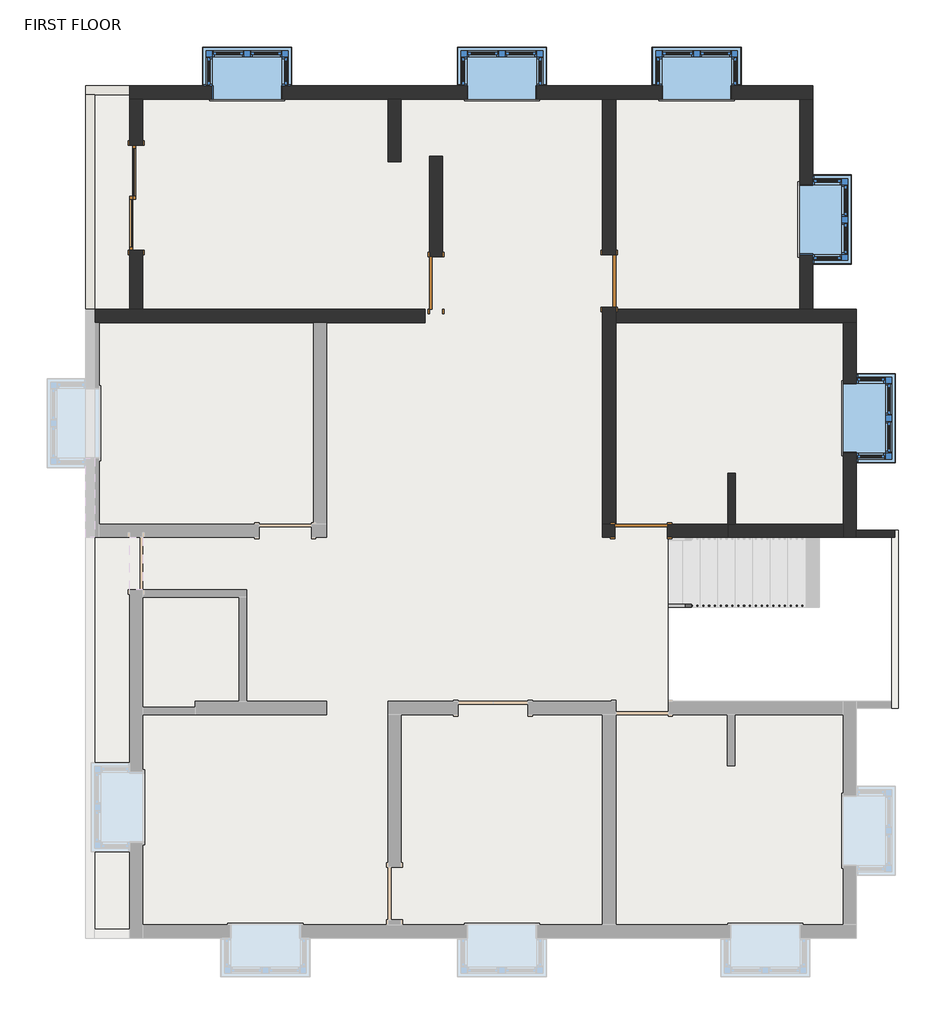
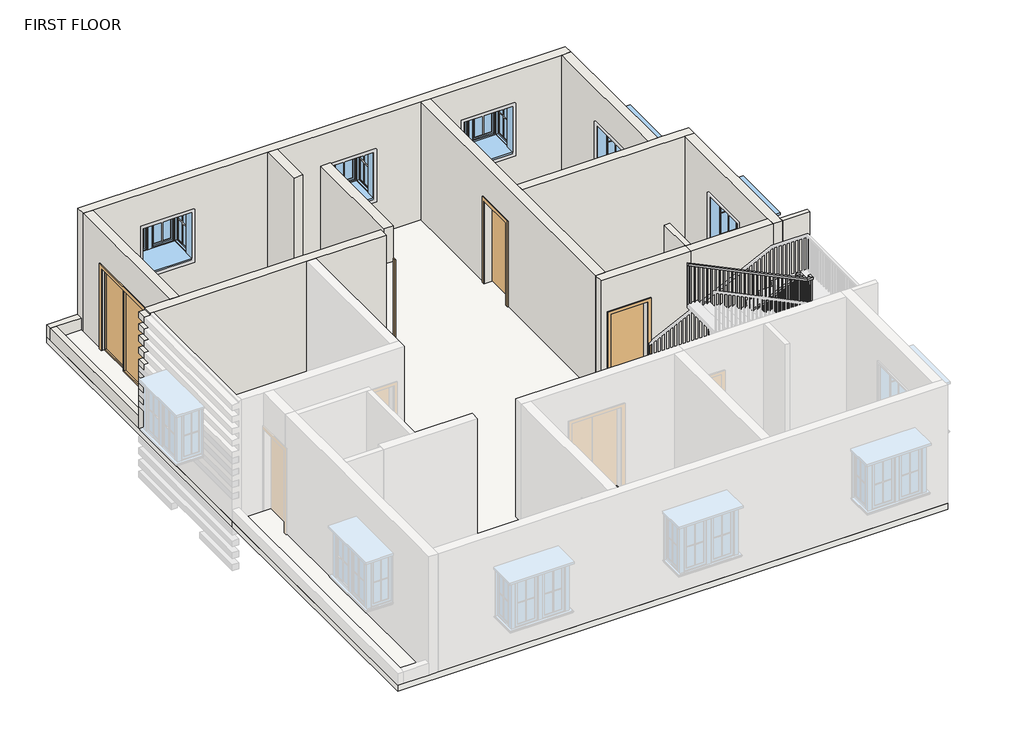
# One storey, part 2 of 6: 15 walls, 5 windows, 4 doors, 1 railing, 1 slab.
"""IFC4 building model written with IfcOpenShell, lengths in millimetres."""

from ifc_helpers import new_model, si_unit, frame, origin, place, context, project, spatial, polyline, outline, extrude, faceted_brep, transform, mapped, element, save
from components import door_d4d75d1e, door_a90ba1ad, door_0ca8825f, window_bay_casement_box_90_degree_angle_4_x4_x2_07b705a1

model = new_model("IFC4")

# Units and contexts
model_context = context("Model", 3, world=origin())
ifc_project = project(units=[si_unit("LENGTHUNIT", "METRE", prefix="MILLI")], contexts=[model_context])

# Site, building, storey
site = spatial("IfcSite", under=ifc_project)
building = spatial("IfcBuilding", under=site)
storey = spatial("IfcBuildingStorey", under=building, Name="FIRST FLOOR", Elevation=3200.4)

# Doors
placement = place(None, origin())
door_shape = door_d4d75d1e(model_context)
element("IfcDoor", 1, ObjectType="Door-Double-Sliding : 72\" x 84\"", at=placement, inside=storey, context=model_context, shape_type="MappedRepresentation", body=[
    mapped(door_shape, transform((-6005.0415084, 6126.233346, 3200.4), x_axis=(0.0, 1.0, 0.0), y_axis=(-1.0, 0.0, 0.0), z_axis=(0.0, 0.0, 1.0))),
])
door_2_shape = door_a90ba1ad(model_context)
element("IfcDoor", 2, ObjectType="Single-Flush : 36\" x 84\"", at=placement, inside=storey, context=model_context, shape_type="MappedRepresentation", body=[
    mapped(door_2_shape, transform((2656.3584916, 335.033346, 3200.4), x_axis=(-1.0, 0.0, 0.0), y_axis=(0.0, -1.0, 0.0), z_axis=(0.0, 0.0, 1.0))),
])
element("IfcDoor", 3, ObjectType="Single-Flush : 36\" x 84\"", at=placement, inside=storey, context=model_context, shape_type="MappedRepresentation", body=[
    mapped(door_2_shape, transform((-918.5024437, 4640.333346, 3200.4), x_axis=(0.0, -1.0, 0.0), y_axis=(1.0, 0.0, 0.0), z_axis=(0.0, 0.0, 1.0))),
])
door_3_shape = door_0ca8825f(model_context)
element("IfcDoor", 4, ObjectType="Single-Flush : 36\" x 84\"", at=placement, inside=storey, context=model_context, shape_type="MappedRepresentation", body=[
    mapped(door_3_shape, transform((2097.5584916, 4678.433346, 3200.4), x_axis=(0.0, -1.0, 0.0), y_axis=(1.0, 0.0, 0.0), z_axis=(0.0, 0.0, 1.0))),
])

# Railing
element("IfcRailing", 5, ObjectType="Handrail - Rectangular", at=placement, inside=storey, context=model_context, shape_type="SolidModel", body=[
    faceted_brep([(3126.2584916, -947.666654, 4260.2727273), (3126.2584916, -947.666654, 4203.7956113), (3126.2584916, -998.466654, 4203.7956113), (3126.2584916, -998.466654, 4260.2727273), (6044.5829507, -947.666654, 5677.9823634), (6095.3829507, -947.666654, 5646.1836718), (6095.3829507, -998.466654, 5646.1836718), (6044.5829507, -998.466654, 5677.9823634), (6044.5829507, -947.666654, 5715.0), (6095.3829507, -947.666654, 5664.2), (6095.3829507, -998.466654, 5664.2), (6044.5829507, -998.466654, 5715.0), (6171.5829507, -947.666654, 5715.0), (6171.5829507, -947.666654, 5664.2), (6120.7829507, -998.466654, 5664.2), (6120.7829507, -998.466654, 5715.0), (6171.5829507, -1074.666654, 5715.0), (6171.5829507, -1074.666654, 5664.2), (6120.7829507, -1074.666654, 5664.2), (6120.7829507, -1074.666654, 5715.0), (6171.5829507, -1341.366654, 5715.0), (6171.5829507, -1392.166654, 5664.2), (6120.7829507, -1392.166654, 5664.2), (6120.7829507, -1341.366654, 5715.0), (6171.5829507, -1341.366654, 5897.4903639), (6171.5829507, -1392.166654, 5846.6903639), (6120.7829507, -1392.166654, 5846.6903639), (6120.7829507, -1341.366654, 5897.4903639), (6171.5829507, -1468.366654, 5897.4903639), (6171.5829507, -1468.366654, 5846.6903639), (6120.7829507, -1417.566654, 5846.6903639), (6120.7829507, -1417.566654, 5897.4903639), (6044.5829507, -1468.366654, 5897.4903639), (6032.8967309, -1468.366654, 5846.6903639), (6032.8967309, -1417.566654, 5846.6903639), (6044.5829507, -1417.566654, 5897.4903639), (3126.2584916, -1468.366654, 7315.2), (3126.2584916, -1417.566654, 7315.2), (3126.2584916, -1417.566654, 7258.722884), (3126.2584916, -1468.366654, 7258.722884)], [[[0, 1, 2, 3]], [[1, 0, 4, 5]], [[2, 1, 5, 6]], [[3, 2, 6, 7]], [[0, 3, 7, 4]], [[5, 4, 8, 9]], [[6, 5, 9, 10]], [[7, 6, 10, 11]], [[4, 7, 11, 8]], [[9, 8, 12, 13]], [[10, 9, 13, 14]], [[11, 10, 14, 15]], [[8, 11, 15, 12]], [[13, 12, 16, 17]], [[14, 13, 17, 18]], [[15, 14, 18, 19]], [[12, 15, 19, 16]], [[17, 16, 20, 21]], [[18, 17, 21, 22]], [[19, 18, 22, 23]], [[16, 19, 23, 20]], [[21, 20, 24, 25]], [[22, 21, 25, 26]], [[23, 22, 26, 27]], [[20, 23, 27, 24]], [[25, 24, 28, 29]], [[26, 25, 29, 30]], [[27, 26, 30, 31]], [[24, 27, 31, 28]], [[29, 28, 32, 33]], [[30, 29, 33, 34]], [[31, 30, 34, 35]], [[28, 31, 35, 32]], [[36, 37, 38, 39]], [[33, 32, 36, 39]], [[34, 33, 39, 38]], [[35, 34, 38, 37]], [[32, 35, 37, 36]]]),
    extrude(outline(polyline([(7218.3778093, 3209.3079507), (7227.6322184, 3190.2579507), (6255.3272727, 3190.2579507), (6255.3272727, 3209.3079507), (7218.3778093, 3209.3079507)])), frame((0.0, -1452.491654, 0.0), z_axis=(0.0, 1.0, 0.0), x_axis=(0.0, 0.0, 1.0)), (0.0, 0.0, 1.0), 19.05),
    extrude(outline(polyline([(7169.0209605, 3310.9079507), (7178.2753696, 3291.8579507), (6255.3272727, 3291.8579507), (6255.3272727, 3310.9079507), (7169.0209605, 3310.9079507)])), frame((0.0, -1452.491654, 0.0), z_axis=(0.0, 1.0, 0.0), x_axis=(0.0, 0.0, 1.0)), (0.0, 0.0, 1.0), 19.05),
    extrude(outline(polyline([(7119.6641117, 3412.5079507), (7128.9185208, 3393.4579507), (6109.8545455, 3393.4579507), (6109.8545455, 3412.5079507), (7119.6641117, 3412.5079507)])), frame((0.0, -1452.491654, 0.0), z_axis=(0.0, 1.0, 0.0), x_axis=(0.0, 0.0, 1.0)), (0.0, 0.0, 1.0), 19.05),
    extrude(outline(polyline([(7070.3072629, 3514.1079507), (7079.5616721, 3495.0579507), (6109.8545455, 3495.0579507), (6109.8545455, 3514.1079507), (7070.3072629, 3514.1079507)])), frame((0.0, -1452.491654, 0.0), z_axis=(0.0, 1.0, 0.0), x_axis=(0.0, 0.0, 1.0)), (0.0, 0.0, 1.0), 19.05),
    extrude(outline(polyline([(7020.9504141, 3615.7079507), (7030.2048233, 3596.6579507), (6109.8545455, 3596.6579507), (6109.8545455, 3615.7079507), (7020.9504141, 3615.7079507)])), frame((0.0, -1452.491654, 0.0), z_axis=(0.0, 1.0, 0.0), x_axis=(0.0, 0.0, 1.0)), (0.0, 0.0, 1.0), 19.05),
    extrude(outline(polyline([(6971.5935653, 3717.3079507), (6980.8479745, 3698.2579507), (5964.3818182, 3698.2579507), (5964.3818182, 3717.3079507), (6971.5935653, 3717.3079507)])), frame((0.0, -1452.491654, 0.0), z_axis=(0.0, 1.0, 0.0), x_axis=(0.0, 0.0, 1.0)), (0.0, 0.0, 1.0), 19.05),
    extrude(outline(polyline([(6922.2367166, 3818.9079507), (6931.4911257, 3799.8579507), (5964.3818182, 3799.8579507), (5964.3818182, 3818.9079507), (6922.2367166, 3818.9079507)])), frame((0.0, -1452.491654, 0.0), z_axis=(0.0, 1.0, 0.0), x_axis=(0.0, 0.0, 1.0)), (0.0, 0.0, 1.0), 19.05),
    extrude(outline(polyline([(6872.8798678, 3920.5079507), (6882.1342769, 3901.4579507), (5964.3818182, 3901.4579507), (5964.3818182, 3920.5079507), (6872.8798678, 3920.5079507)])), frame((0.0, -1452.491654, 0.0), z_axis=(0.0, 1.0, 0.0), x_axis=(0.0, 0.0, 1.0)), (0.0, 0.0, 1.0), 19.05),
    extrude(outline(polyline([(6823.523019, 4022.1079507), (6832.7774281, 4003.0579507), (5818.9090909, 4003.0579507), (5818.9090909, 4022.1079507), (6823.523019, 4022.1079507)])), frame((0.0, -1452.491654, 0.0), z_axis=(0.0, 1.0, 0.0), x_axis=(0.0, 0.0, 1.0)), (0.0, 0.0, 1.0), 19.05),
    extrude(outline(polyline([(6774.1661702, 4123.7079507), (6783.4205793, 4104.6579507), (5818.9090909, 4104.6579507), (5818.9090909, 4123.7079507), (6774.1661702, 4123.7079507)])), frame((0.0, -1452.491654, 0.0), z_axis=(0.0, 1.0, 0.0), x_axis=(0.0, 0.0, 1.0)), (0.0, 0.0, 1.0), 19.05),
    extrude(outline(polyline([(6724.8093214, 4225.3079507), (6734.0637306, 4206.2579507), (5818.9090909, 4206.2579507), (5818.9090909, 4225.3079507), (6724.8093214, 4225.3079507)])), frame((0.0, -1452.491654, 0.0), z_axis=(0.0, 1.0, 0.0), x_axis=(0.0, 0.0, 1.0)), (0.0, 0.0, 1.0), 19.05),
    extrude(outline(polyline([(6675.4524726, 4326.9079507), (6684.7068818, 4307.8579507), (5673.4363636, 4307.8579507), (5673.4363636, 4326.9079507), (6675.4524726, 4326.9079507)])), frame((0.0, -1452.491654, 0.0), z_axis=(0.0, 1.0, 0.0), x_axis=(0.0, 0.0, 1.0)), (0.0, 0.0, 1.0), 19.05),
    extrude(outline(polyline([(6626.0956238, 4428.5079507), (6635.350033, 4409.4579507), (5673.4363636, 4409.4579507), (5673.4363636, 4428.5079507), (6626.0956238, 4428.5079507)])), frame((0.0, -1452.491654, 0.0), z_axis=(0.0, 1.0, 0.0), x_axis=(0.0, 0.0, 1.0)), (0.0, 0.0, 1.0), 19.05),
    extrude(outline(polyline([(6576.7387751, 4530.1079507), (6585.9931842, 4511.0579507), (5673.4363636, 4511.0579507), (5673.4363636, 4530.1079507), (6576.7387751, 4530.1079507)])), frame((0.0, -1452.491654, 0.0), z_axis=(0.0, 1.0, 0.0), x_axis=(0.0, 0.0, 1.0)), (0.0, 0.0, 1.0), 19.05),
    extrude(outline(polyline([(6527.3819263, 4631.7079507), (6536.6363354, 4612.6579507), (5527.9636364, 4612.6579507), (5527.9636364, 4631.7079507), (6527.3819263, 4631.7079507)])), frame((0.0, -1452.491654, 0.0), z_axis=(0.0, 1.0, 0.0), x_axis=(0.0, 0.0, 1.0)), (0.0, 0.0, 1.0), 19.05),
    extrude(outline(polyline([(6478.0250775, 4733.3079507), (6487.2794866, 4714.2579507), (5527.9636364, 4714.2579507), (5527.9636364, 4733.3079507), (6478.0250775, 4733.3079507)])), frame((0.0, -1452.491654, 0.0), z_axis=(0.0, 1.0, 0.0), x_axis=(0.0, 0.0, 1.0)), (0.0, 0.0, 1.0), 19.05),
    extrude(outline(polyline([(6428.6682287, 4834.9079507), (6437.9226379, 4815.8579507), (5527.9636364, 4815.8579507), (5527.9636364, 4834.9079507), (6428.6682287, 4834.9079507)])), frame((0.0, -1452.491654, 0.0), z_axis=(0.0, 1.0, 0.0), x_axis=(0.0, 0.0, 1.0)), (0.0, 0.0, 1.0), 19.05),
    extrude(outline(polyline([(6379.3113799, 4936.5079507), (6388.5657891, 4917.4579507), (5382.4909091, 4917.4579507), (5382.4909091, 4936.5079507), (6379.3113799, 4936.5079507)])), frame((0.0, -1452.491654, 0.0), z_axis=(0.0, 1.0, 0.0), x_axis=(0.0, 0.0, 1.0)), (0.0, 0.0, 1.0), 19.05),
    extrude(outline(polyline([(6329.9545311, 5038.1079507), (6339.2089403, 5019.0579507), (5382.4909091, 5019.0579507), (5382.4909091, 5038.1079507), (6329.9545311, 5038.1079507)])), frame((0.0, -1452.491654, 0.0), z_axis=(0.0, 1.0, 0.0), x_axis=(0.0, 0.0, 1.0)), (0.0, 0.0, 1.0), 19.05),
    extrude(outline(polyline([(6280.5976824, 5139.7079507), (6289.8520915, 5120.6579507), (5382.4909091, 5120.6579507), (5382.4909091, 5139.7079507), (6280.5976824, 5139.7079507)])), frame((0.0, -1452.491654, 0.0), z_axis=(0.0, 1.0, 0.0), x_axis=(0.0, 0.0, 1.0)), (0.0, 0.0, 1.0), 19.05),
    extrude(outline(polyline([(6231.159384, 5241.3079507), (6240.4137931, 5222.2579507), (5237.0181818, 5222.2579507), (5237.0181818, 5241.3079507), (6231.159384, 5241.3079507)])), frame((0.0, -1452.491654, 0.0), z_axis=(0.0, 1.0, 0.0), x_axis=(0.0, 0.0, 1.0)), (0.0, 0.0, 1.0), 19.05),
    extrude(outline(polyline([(6181.8839848, 5342.9079507), (6191.1383939, 5323.8579507), (5237.0181818, 5323.8579507), (5237.0181818, 5342.9079507), (6181.8839848, 5342.9079507)])), frame((0.0, -1452.491654, 0.0), z_axis=(0.0, 1.0, 0.0), x_axis=(0.0, 0.0, 1.0)), (0.0, 0.0, 1.0), 19.05),
    extrude(outline(polyline([(6132.527136, 5444.5079507), (6141.7815452, 5425.4579507), (5237.0181818, 5425.4579507), (5237.0181818, 5444.5079507), (6132.527136, 5444.5079507)])), frame((0.0, -1452.491654, 0.0), z_axis=(0.0, 1.0, 0.0), x_axis=(0.0, 0.0, 1.0)), (0.0, 0.0, 1.0), 19.05),
    extrude(outline(polyline([(6083.1702872, 5546.1079507), (6092.4246964, 5527.0579507), (5091.5454545, 5527.0579507), (5091.5454545, 5546.1079507), (6083.1702872, 5546.1079507)])), frame((0.0, -1452.491654, 0.0), z_axis=(0.0, 1.0, 0.0), x_axis=(0.0, 0.0, 1.0)), (0.0, 0.0, 1.0), 19.05),
    extrude(outline(polyline([(6033.8134384, 5647.7079507), (6043.0678476, 5628.6579507), (5091.5454545, 5628.6579507), (5091.5454545, 5647.7079507), (6033.8134384, 5647.7079507)])), frame((0.0, -1452.491654, 0.0), z_axis=(0.0, 1.0, 0.0), x_axis=(0.0, 0.0, 1.0)), (0.0, 0.0, 1.0), 19.05),
    extrude(outline(polyline([(5984.4565897, 5749.3079507), (5993.7109988, 5730.2579507), (5091.5454545, 5730.2579507), (5091.5454545, 5749.3079507), (5984.4565897, 5749.3079507)])), frame((0.0, -1452.491654, 0.0), z_axis=(0.0, 1.0, 0.0), x_axis=(0.0, 0.0, 1.0)), (0.0, 0.0, 1.0), 19.05),
    extrude(outline(polyline([(5935.0997409, 5850.9079507), (5944.35415, 5831.8579507), (4946.0727273, 5831.8579507), (4946.0727273, 5850.9079507), (5935.0997409, 5850.9079507)])), frame((0.0, -1452.491654, 0.0), z_axis=(0.0, 1.0, 0.0), x_axis=(0.0, 0.0, 1.0)), (0.0, 0.0, 1.0), 19.05),
    extrude(outline(polyline([(5885.7428921, 5952.5079507), (5894.9973012, 5933.4579507), (4946.0727273, 5933.4579507), (4946.0727273, 5952.5079507), (5885.7428921, 5952.5079507)])), frame((0.0, -1452.491654, 0.0), z_axis=(0.0, 1.0, 0.0), x_axis=(0.0, 0.0, 1.0)), (0.0, 0.0, 1.0), 19.05),
    extrude(outline(polyline([(5836.3860433, 6054.1079507), (5845.6404524, 6035.0579507), (4946.0727273, 6035.0579507), (4946.0727273, 6054.1079507), (5836.3860433, 6054.1079507)])), frame((0.0, -1452.491654, 0.0), z_axis=(0.0, 1.0, 0.0), x_axis=(0.0, 0.0, 1.0)), (0.0, 0.0, 1.0), 19.05),
    extrude(outline(polyline([(6136.6579507, -1369.941654), (6155.7079507, -1369.941654), (6155.7079507, -1388.991654), (6136.6579507, -1388.991654), (6136.6579507, -1369.941654)])), frame((0.0, 0.0, 4800.6), z_axis=(0.0, 0.0, 1.0), x_axis=(1.0, 0.0, 0.0)), (0.0, 0.0, 1.0), 1046.0903639),
    extrude(outline(polyline([(6136.6579507, -1268.341654), (6155.7079507, -1268.341654), (6155.7079507, -1287.391654), (6136.6579507, -1287.391654), (6136.6579507, -1268.341654)])), frame((0.0, 0.0, 4800.6), z_axis=(0.0, 0.0, 1.0), x_axis=(1.0, 0.0, 0.0)), (0.0, 0.0, 1.0), 863.6),
    extrude(outline(polyline([(6136.6579507, -1166.741654), (6155.7079507, -1166.741654), (6155.7079507, -1185.791654), (6136.6579507, -1185.791654), (6136.6579507, -1166.741654)])), frame((0.0, 0.0, 4800.6), z_axis=(0.0, 0.0, 1.0), x_axis=(1.0, 0.0, 0.0)), (0.0, 0.0, 1.0), 863.6),
    extrude(outline(polyline([(6136.6579507, -1065.141654), (6155.7079507, -1065.141654), (6155.7079507, -1084.191654), (6136.6579507, -1084.191654), (6136.6579507, -1065.141654)])), frame((0.0, 0.0, 4800.6), z_axis=(0.0, 0.0, 1.0), x_axis=(1.0, 0.0, 0.0)), (0.0, 0.0, 1.0), 863.6),
    extrude(outline(polyline([(6063.1334916, -982.591654), (6063.1334916, -963.541654), (6082.1834916, -963.541654), (6082.1834916, -982.591654), (6063.1334916, -982.591654)])), frame((0.0, 0.0, 4655.1272727), z_axis=(0.0, 0.0, 1.0), x_axis=(1.0, 0.0, 0.0)), (0.0, 0.0, 1.0), 1009.0727273),
    extrude(outline(polyline([(5590.4145818, 5980.5834916), (5581.1601727, 5961.5334916), (4655.1272727, 5961.5334916), (4655.1272727, 5980.5834916), (5590.4145818, 5980.5834916)])), frame((0.0, -982.591654, 0.0), z_axis=(0.0, 1.0, 0.0), x_axis=(0.0, 0.0, 1.0)), (0.0, 0.0, 1.0), 19.05),
    extrude(outline(polyline([(5541.057733, 5878.9834916), (5531.8033239, 5859.9334916), (4655.1272727, 5859.9334916), (4655.1272727, 5878.9834916), (5541.057733, 5878.9834916)])), frame((0.0, -982.591654, 0.0), z_axis=(0.0, 1.0, 0.0), x_axis=(0.0, 0.0, 1.0)), (0.0, 0.0, 1.0), 19.05),
    extrude(outline(polyline([(5491.7008843, 5777.3834916), (5482.4464751, 5758.3334916), (4509.6545455, 5758.3334916), (4509.6545455, 5777.3834916), (5491.7008843, 5777.3834916)])), frame((0.0, -982.591654, 0.0), z_axis=(0.0, 1.0, 0.0), x_axis=(0.0, 0.0, 1.0)), (0.0, 0.0, 1.0), 19.05),
    extrude(outline(polyline([(5442.3440355, 5675.7834916), (5433.0896263, 5656.7334916), (4509.6545455, 5656.7334916), (4509.6545455, 5675.7834916), (5442.3440355, 5675.7834916)])), frame((0.0, -982.591654, 0.0), z_axis=(0.0, 1.0, 0.0), x_axis=(0.0, 0.0, 1.0)), (0.0, 0.0, 1.0), 19.05),
    extrude(outline(polyline([(5392.9871867, 5574.1834916), (5383.7327775, 5555.1334916), (4509.6545455, 5555.1334916), (4509.6545455, 5574.1834916), (5392.9871867, 5574.1834916)])), frame((0.0, -982.591654, 0.0), z_axis=(0.0, 1.0, 0.0), x_axis=(0.0, 0.0, 1.0)), (0.0, 0.0, 1.0), 19.05),
    extrude(outline(polyline([(5343.6303379, 5472.5834916), (5334.3759288, 5453.5334916), (4364.1818182, 5453.5334916), (4364.1818182, 5472.5834916), (5343.6303379, 5472.5834916)])), frame((0.0, -982.591654, 0.0), z_axis=(0.0, 1.0, 0.0), x_axis=(0.0, 0.0, 1.0)), (0.0, 0.0, 1.0), 19.05),
    extrude(outline(polyline([(5294.2734891, 5370.9834916), (5285.01908, 5351.9334916), (4364.1818182, 5351.9334916), (4364.1818182, 5370.9834916), (5294.2734891, 5370.9834916)])), frame((0.0, -982.591654, 0.0), z_axis=(0.0, 1.0, 0.0), x_axis=(0.0, 0.0, 1.0)), (0.0, 0.0, 1.0), 19.05),
    extrude(outline(polyline([(5244.9166403, 5269.3834916), (5235.6622312, 5250.3334916), (4364.1818182, 5250.3334916), (4364.1818182, 5269.3834916), (5244.9166403, 5269.3834916)])), frame((0.0, -982.591654, 0.0), z_axis=(0.0, 1.0, 0.0), x_axis=(0.0, 0.0, 1.0)), (0.0, 0.0, 1.0), 19.05),
    extrude(outline(polyline([(5195.5597915, 5167.7834916), (5186.3053824, 5148.7334916), (4218.7090909, 5148.7334916), (4218.7090909, 5167.7834916), (5195.5597915, 5167.7834916)])), frame((0.0, -982.591654, 0.0), z_axis=(0.0, 1.0, 0.0), x_axis=(0.0, 0.0, 1.0)), (0.0, 0.0, 1.0), 19.05),
    extrude(outline(polyline([(5146.2029428, 5066.1834916), (5136.9485336, 5047.1334916), (4218.7090909, 5047.1334916), (4218.7090909, 5066.1834916), (5146.2029428, 5066.1834916)])), frame((0.0, -982.591654, 0.0), z_axis=(0.0, 1.0, 0.0), x_axis=(0.0, 0.0, 1.0)), (0.0, 0.0, 1.0), 19.05),
    extrude(outline(polyline([(5096.846094, 4964.5834916), (5087.5916848, 4945.5334916), (4218.7090909, 4945.5334916), (4218.7090909, 4964.5834916), (5096.846094, 4964.5834916)])), frame((0.0, -982.591654, 0.0), z_axis=(0.0, 1.0, 0.0), x_axis=(0.0, 0.0, 1.0)), (0.0, 0.0, 1.0), 19.05),
    extrude(outline(polyline([(5047.4892452, 4862.9834916), (5038.234836, 4843.9334916), (4073.2363636, 4843.9334916), (4073.2363636, 4862.9834916), (5047.4892452, 4862.9834916)])), frame((0.0, -982.591654, 0.0), z_axis=(0.0, 1.0, 0.0), x_axis=(0.0, 0.0, 1.0)), (0.0, 0.0, 1.0), 19.05),
    extrude(outline(polyline([(4998.1323964, 4761.3834916), (4988.8779873, 4742.3334916), (4073.2363636, 4742.3334916), (4073.2363636, 4761.3834916), (4998.1323964, 4761.3834916)])), frame((0.0, -982.591654, 0.0), z_axis=(0.0, 1.0, 0.0), x_axis=(0.0, 0.0, 1.0)), (0.0, 0.0, 1.0), 19.05),
    extrude(outline(polyline([(4948.7755476, 4659.7834916), (4939.5211385, 4640.7334916), (4073.2363636, 4640.7334916), (4073.2363636, 4659.7834916), (4948.7755476, 4659.7834916)])), frame((0.0, -982.591654, 0.0), z_axis=(0.0, 1.0, 0.0), x_axis=(0.0, 0.0, 1.0)), (0.0, 0.0, 1.0), 19.05),
    extrude(outline(polyline([(4899.4186988, 4558.1834916), (4890.1642897, 4539.1334916), (3927.7636364, 4539.1334916), (3927.7636364, 4558.1834916), (4899.4186988, 4558.1834916)])), frame((0.0, -982.591654, 0.0), z_axis=(0.0, 1.0, 0.0), x_axis=(0.0, 0.0, 1.0)), (0.0, 0.0, 1.0), 19.05),
    extrude(outline(polyline([(4850.0618501, 4456.5834916), (4840.8074409, 4437.5334916), (3927.7636364, 4437.5334916), (3927.7636364, 4456.5834916), (4850.0618501, 4456.5834916)])), frame((0.0, -982.591654, 0.0), z_axis=(0.0, 1.0, 0.0), x_axis=(0.0, 0.0, 1.0)), (0.0, 0.0, 1.0), 19.05),
    extrude(outline(polyline([(4800.7050013, 4354.9834916), (4791.4505921, 4335.9334916), (3927.7636364, 4335.9334916), (3927.7636364, 4354.9834916), (4800.7050013, 4354.9834916)])), frame((0.0, -982.591654, 0.0), z_axis=(0.0, 1.0, 0.0), x_axis=(0.0, 0.0, 1.0)), (0.0, 0.0, 1.0), 19.05),
    extrude(outline(polyline([(4751.3481525, 4253.3834916), (4742.0937433, 4234.3334916), (3782.2909091, 4234.3334916), (3782.2909091, 4253.3834916), (4751.3481525, 4253.3834916)])), frame((0.0, -982.591654, 0.0), z_axis=(0.0, 1.0, 0.0), x_axis=(0.0, 0.0, 1.0)), (0.0, 0.0, 1.0), 19.05),
    extrude(outline(polyline([(4701.9913037, 4151.7834916), (4692.7368946, 4132.7334916), (3782.2909091, 4132.7334916), (3782.2909091, 4151.7834916), (4701.9913037, 4151.7834916)])), frame((0.0, -982.591654, 0.0), z_axis=(0.0, 1.0, 0.0), x_axis=(0.0, 0.0, 1.0)), (0.0, 0.0, 1.0), 19.05),
    extrude(outline(polyline([(4652.6344549, 4050.1834916), (4643.3800458, 4031.1334916), (3782.2909091, 4031.1334916), (3782.2909091, 4050.1834916), (4652.6344549, 4050.1834916)])), frame((0.0, -982.591654, 0.0), z_axis=(0.0, 1.0, 0.0), x_axis=(0.0, 0.0, 1.0)), (0.0, 0.0, 1.0), 19.05),
    extrude(outline(polyline([(4603.2776061, 3948.5834916), (4594.023197, 3929.5334916), (3636.8181818, 3929.5334916), (3636.8181818, 3948.5834916), (4603.2776061, 3948.5834916)])), frame((0.0, -982.591654, 0.0), z_axis=(0.0, 1.0, 0.0), x_axis=(0.0, 0.0, 1.0)), (0.0, 0.0, 1.0), 19.05),
    extrude(outline(polyline([(4553.9207573, 3846.9834916), (4544.6663482, 3827.9334916), (3636.8181818, 3827.9334916), (3636.8181818, 3846.9834916), (4553.9207573, 3846.9834916)])), frame((0.0, -982.591654, 0.0), z_axis=(0.0, 1.0, 0.0), x_axis=(0.0, 0.0, 1.0)), (0.0, 0.0, 1.0), 19.05),
    extrude(outline(polyline([(4504.5639086, 3745.3834916), (4495.3094994, 3726.3334916), (3636.8181818, 3726.3334916), (3636.8181818, 3745.3834916), (4504.5639086, 3745.3834916)])), frame((0.0, -982.591654, 0.0), z_axis=(0.0, 1.0, 0.0), x_axis=(0.0, 0.0, 1.0)), (0.0, 0.0, 1.0), 19.05),
    extrude(outline(polyline([(4455.2070598, 3643.7834916), (4445.9526506, 3624.7334916), (3491.3454545, 3624.7334916), (3491.3454545, 3643.7834916), (4455.2070598, 3643.7834916)])), frame((0.0, -982.591654, 0.0), z_axis=(0.0, 1.0, 0.0), x_axis=(0.0, 0.0, 1.0)), (0.0, 0.0, 1.0), 19.05),
    extrude(outline(polyline([(4405.850211, 3542.1834916), (4396.5958018, 3523.1334916), (3491.3454545, 3523.1334916), (3491.3454545, 3542.1834916), (4405.850211, 3542.1834916)])), frame((0.0, -982.591654, 0.0), z_axis=(0.0, 1.0, 0.0), x_axis=(0.0, 0.0, 1.0)), (0.0, 0.0, 1.0), 19.05),
    extrude(outline(polyline([(4356.4933622, 3440.5834916), (4347.2389531, 3421.5334916), (3491.3454545, 3421.5334916), (3491.3454545, 3440.5834916), (4356.4933622, 3440.5834916)])), frame((0.0, -982.591654, 0.0), z_axis=(0.0, 1.0, 0.0), x_axis=(0.0, 0.0, 1.0)), (0.0, 0.0, 1.0), 19.05),
    extrude(outline(polyline([(4307.1365134, 3338.9834916), (4297.8821043, 3319.9334916), (3345.8727273, 3319.9334916), (3345.8727273, 3338.9834916), (4307.1365134, 3338.9834916)])), frame((0.0, -982.591654, 0.0), z_axis=(0.0, 1.0, 0.0), x_axis=(0.0, 0.0, 1.0)), (0.0, 0.0, 1.0), 19.05),
    extrude(outline(polyline([(4257.7796646, 3237.3834916), (4248.5252555, 3218.3334916), (3345.8727273, 3218.3334916), (3345.8727273, 3237.3834916), (4257.7796646, 3237.3834916)])), frame((0.0, -982.591654, 0.0), z_axis=(0.0, 1.0, 0.0), x_axis=(0.0, 0.0, 1.0)), (0.0, 0.0, 1.0), 19.05),
    extrude(outline(polyline([(6136.6579507, -1433.441654), (6155.7079507, -1433.441654), (6155.7079507, -1452.491654), (6136.6579507, -1452.491654), (6136.6579507, -1433.441654)])), frame((0.0, 0.0, 4800.6), z_axis=(0.0, 0.0, 1.0), x_axis=(1.0, 0.0, 0.0)), (0.0, 0.0, 1.0), 1046.0903639),
    extrude(outline(polyline([(6136.6579507, -982.591654), (6136.6579507, -963.541654), (6155.7079507, -963.541654), (6155.7079507, -982.591654), (6136.6579507, -982.591654)])), frame((0.0, 0.0, 4800.6), z_axis=(0.0, 0.0, 1.0), x_axis=(1.0, 0.0, 0.0)), (0.0, 0.0, 1.0), 863.6),
    extrude(outline(polyline([(7249.4684749, 3145.3084916), (7258.722884, 3126.2584916), (6255.3272727, 3126.2584916), (6255.3272727, 3145.3084916), (7249.4684749, 3145.3084916)])), frame((0.0, -1452.491654, 0.0), z_axis=(0.0, 1.0, 0.0), x_axis=(0.0, 0.0, 1.0)), (0.0, 0.0, 1.0), 19.05),
    extrude(outline(polyline([(4213.0500204, 3145.3084916), (4203.7956113, 3126.2584916), (3345.8727273, 3126.2584916), (3345.8727273, 3145.3084916), (4213.0500204, 3145.3084916)])), frame((0.0, -982.591654, 0.0), z_axis=(0.0, 1.0, 0.0), x_axis=(0.0, 0.0, 1.0)), (0.0, 0.0, 1.0), 19.05),
])

# Slab
element("IfcSlab", 6, ObjectType="6\"", at=placement, inside=storey, context=model_context, shape_type="SweptSolid", body=[
    extrude(outline(polyline([(-7008.3415084, -6751.566654), (-7008.3415084, 220.733346), (-7008.3415084, 8069.333346), (5640.8584916, 8069.333346), (5640.8584916, 4183.133346), (6402.8584916, 4183.133346), (6402.8584916, 337.573346), (7125.9750459, 337.573346), (7125.9750459, -2753.606654), (6402.8584916, -2753.606654), (6402.8584916, -6751.566654), (-7008.3415084, -6751.566654)]), holes=[polyline([(7009.1350459, 220.733346), (3126.2584916, 220.733346), (3126.2584916, -2636.766654), (7009.1350459, -2636.766654), (7009.1350459, 220.733346)])]), frame((0.0, 0.0, 3048.0), z_axis=(0.0, 0.0, 1.0), x_axis=(1.0, 0.0, 0.0)), (0.0, 0.0, 1.0), 152.4),
])

# Walls
element("IfcWall", 7, ObjectType="4.6\"", at=placement, inside=storey, context=model_context, shape_type="SweptSolid", body=[
    extrude(outline(polyline([(7067.5550459, 220.733346), (6402.8584916, 220.733346), (6402.8584916, 337.573346), (7067.5550459, 337.573346), (7067.5550459, 220.733346)])), frame((0.0, 0.0, 3200.4), z_axis=(0.0, 0.0, 1.0), x_axis=(1.0, 0.0, 0.0)), (0.0, 0.0, 1.0), 3048.0),
])
element("IfcWall", 8, ObjectType="5\"", at=placement, inside=storey, context=model_context, shape_type="SweptSolid", body=[
    extrude(outline(polyline([(4291.9829507, 1335.1417393), (4291.9829507, 449.333346), (4164.9829507, 449.333346), (4164.9829507, 1335.1417393), (4291.9829507, 1335.1417393)])), frame((0.0, 0.0, 3200.4), z_axis=(0.0, 0.0, 1.0), x_axis=(1.0, 0.0, 0.0)), (0.0, 0.0, 1.0), 3048.0),
])
element("IfcWall", 9, ObjectType="6\"", at=placement, inside=storey, context=model_context, shape_type="Brep", body=[
    faceted_brep([(-6246.3415084, 8069.333346, 3200.4), (-7008.3415084, 8069.333346, 3200.4), (-7008.3415084, 8069.333346, 3505.2), (-6246.3415084, 8069.333346, 3505.2), (-6246.3415084, 7916.933346, 3200.4), (-6246.3415084, 7916.933346, 3505.2), (-6855.9415084, 7916.933346, 3505.2), (-7008.3415084, 7916.933346, 3505.2), (-7008.3415084, 7916.933346, 3200.4), (-6855.9415084, 7916.933346, 3200.4)], [[[0, 1, 2, 3]], [[4, 5, 6, 7, 8, 9]], [[1, 0, 4, 9, 8]], [[3, 2, 7, 6, 5]], [[0, 3, 5, 4]], [[2, 1, 8, 7]]]),
])
element("IfcWall", 10, ObjectType="6\"", at=placement, inside=storey, context=model_context, shape_type="SweptSolid", body=[
    extrude(outline(polyline([(-7008.3415084, 4183.133346), (-7008.3415084, 7916.933346), (-6855.9415084, 7916.933346), (-6855.9415084, 4183.133346), (-7008.3415084, 4183.133346)])), frame((0.0, 0.0, 3200.4), z_axis=(0.0, 0.0, 1.0), x_axis=(1.0, 0.0, 0.0)), (0.0, 0.0, 1.0), 304.8),
])
element("IfcWall", 11, ObjectType="9\"", at=placement, inside=storey, context=model_context, shape_type="Brep", body=[
    faceted_brep([(5640.8584916, 8069.333346, 3200.4), (-6246.3415084, 8069.333346, 3200.4), (-6246.3415084, 8069.333346, 3505.2), (-6246.3415084, 8069.333346, 6248.4), (5640.8584916, 8069.333346, 6248.4), (-3592.0415084, 8069.333346, 5384.8), (-4811.2415084, 8069.333346, 5384.8), (-4811.2415084, 8069.333346, 4114.8), (-3592.0415084, 8069.333346, 4114.8), (4231.1584916, 8069.333346, 5384.8), (3011.9584916, 8069.333346, 5384.8), (3011.9584916, 8069.333346, 4114.8), (4231.1584916, 8069.333346, 4114.8), (840.2584916, 8069.333346, 5384.8), (-378.9415084, 8069.333346, 5384.8), (-378.9415084, 8069.333346, 4114.8), (840.2584916, 8069.333346, 4114.8), (5640.8584916, 7840.733346, 3200.4), (5640.8584916, 7840.733346, 6248.4), (5412.2584916, 7840.733346, 6248.4), (2211.8584916, 7840.733346, 6248.4), (1983.2584916, 7840.733346, 6248.4), (-1521.9415084, 7840.733346, 6248.4), (-1750.5415084, 7840.733346, 6248.4), (-6017.7415084, 7840.733346, 6248.4), (-6246.3415084, 7840.733346, 6248.4), (-6246.3415084, 7840.733346, 3200.4), (-6017.7415084, 7840.733346, 3200.4), (-1750.5415084, 7840.733346, 3200.4), (-1521.9415084, 7840.733346, 3200.4), (1983.2584916, 7840.733346, 3200.4), (2211.8584916, 7840.733346, 3200.4), (5412.2584916, 7840.733346, 3200.4), (-3592.0415084, 7840.733346, 5384.8), (-3592.0415084, 7840.733346, 4114.8), (-4811.2415084, 7840.733346, 4114.8), (-4811.2415084, 7840.733346, 5384.8), (4231.1584916, 7840.733346, 5384.8), (4231.1584916, 7840.733346, 4114.8), (3011.9584916, 7840.733346, 4114.8), (3011.9584916, 7840.733346, 5384.8), (840.2584916, 7840.733346, 5384.8), (840.2584916, 7840.733346, 4114.8), (-378.9415084, 7840.733346, 4114.8), (-378.9415084, 7840.733346, 5384.8), (-6246.3415084, 7916.933346, 3200.4)], [[[0, 1, 2, 3, 4], [5, 6, 7, 8], [9, 10, 11, 12], [13, 14, 15, 16]], [[17, 18, 19, 20, 21, 22, 23, 24, 25, 26, 27, 28, 29, 30, 31, 32], [33, 34, 35, 36], [37, 38, 39, 40], [41, 42, 43, 44]], [[1, 0, 17, 32, 31, 30, 29, 28, 27, 26, 45]], [[4, 3, 25, 24, 23, 22, 21, 20, 19, 18]], [[0, 4, 18, 17]], [[34, 33, 5, 8]], [[35, 34, 8, 7]], [[36, 35, 7, 6]], [[33, 36, 6, 5]], [[38, 37, 9, 12]], [[39, 38, 12, 11]], [[40, 39, 11, 10]], [[37, 40, 10, 9]], [[42, 41, 13, 16]], [[43, 42, 16, 15]], [[44, 43, 15, 14]], [[41, 44, 14, 13]], [[1, 45, 26, 25, 3, 2]]]),
])
element("IfcWall", 12, ObjectType="9\"", at=placement, inside=storey, context=model_context, shape_type="SweptSolid", body=[
    extrude(outline(polyline([(7840.733346, 3200.4), (7040.633346, 3200.4), (7040.633346, 5334.0), (5211.833346, 5334.0), (5211.833346, 3200.4), (4183.133346, 3200.4), (4183.133346, 6248.4), (7840.733346, 6248.4), (7840.733346, 3200.4)])), frame((-6246.3415084, 0.0, 0.0), z_axis=(1.0, 0.0, 0.0), x_axis=(0.0, 1.0, 0.0)), (0.0, 0.0, 1.0), 228.6),
])
element("IfcWall", 13, ObjectType="9\"", at=placement, inside=storey, context=model_context, shape_type="SweptSolid", body=[
    extrude(outline(polyline([(7840.733346, 3200.4), (4183.133346, 3200.4), (4183.133346, 6248.4), (7840.733346, 6248.4), (7840.733346, 3200.4)]), holes=[polyline([(5135.633346, 5384.8), (5135.633346, 4114.8), (6354.833346, 4114.8), (6354.833346, 5384.8), (5135.633346, 5384.8)])]), frame((5412.2584916, 0.0, 0.0), z_axis=(1.0, 0.0, 0.0), x_axis=(0.0, 1.0, 0.0)), (0.0, 0.0, 1.0), 228.6),
])
element("IfcWall", 14, ObjectType="9\"", at=placement, inside=storey, context=model_context, shape_type="Brep", body=[
    faceted_brep([(1983.2584916, 4221.233346, 5334.0), (1983.2584916, 4221.233346, 3200.4), (1983.2584916, 449.333346, 3200.4), (1983.2584916, 449.333346, 6248.4), (1983.2584916, 7840.733346, 6248.4), (1983.2584916, 7840.733346, 3200.4), (1983.2584916, 5135.633346, 3200.4), (1983.2584916, 5135.633346, 5334.0), (2211.8584916, 449.333346, 3200.4), (2211.8584916, 3954.533346, 3200.4), (2211.8584916, 4183.133346, 3200.4), (2211.8584916, 4221.233346, 3200.4), (2211.8584916, 4221.233346, 5334.0), (2211.8584916, 5135.633346, 5334.0), (2211.8584916, 5135.633346, 3200.4), (2211.8584916, 7840.733346, 3200.4), (2211.8584916, 7840.733346, 6248.4), (2211.8584916, 4183.133346, 6248.4), (2211.8584916, 3954.533346, 6248.4), (2211.8584916, 449.333346, 6248.4), (2199.1584916, 449.333346, 3200.4)], [[[0, 1, 2, 3, 4, 5, 6, 7]], [[8, 9, 10, 11, 12, 13, 14, 15, 16, 17, 18, 19]], [[6, 5, 15, 14]], [[2, 1, 11, 10, 9, 8, 20]], [[4, 3, 19, 18, 17, 16]], [[5, 4, 16, 15]], [[3, 2, 20, 8, 19]], [[12, 11, 1, 0]], [[13, 12, 0, 7]], [[14, 13, 7, 6]]]),
])
element("IfcWall", 15, ObjectType="9\"", at=placement, inside=storey, context=model_context, shape_type="SweptSolid", body=[
    extrude(outline(polyline([(-1750.5415084, 6747.0175593), (-1750.5415084, 7840.733346), (-1521.9415084, 7840.733346), (-1521.9415084, 6747.0175593), (-1750.5415084, 6747.0175593)])), frame((0.0, 0.0, 3200.4), z_axis=(0.0, 0.0, 1.0), x_axis=(1.0, 0.0, 0.0)), (0.0, 0.0, 1.0), 3048.0),
])
element("IfcWall", 16, ObjectType="9\"", at=placement, inside=storey, context=model_context, shape_type="Brep", body=[
    faceted_brep([(-1108.4404612, 4183.133346, 3200.4), (-6017.7415084, 4183.133346, 3200.4), (-6246.3415084, 4183.133346, 3200.4), (-6855.9415084, 4183.133346, 3200.4), (-7008.3415084, 4183.133346, 3200.4), (-7008.3415084, 4183.133346, 3505.2), (-7008.3415084, 4183.133346, 3759.2), (-6855.9415084, 4183.133346, 3759.2), (-6855.9415084, 4183.133346, 3911.6), (-7008.3415084, 4183.133346, 3911.6), (-7008.3415084, 4183.133346, 4064.0), (-6855.9415084, 4183.133346, 4064.0), (-6855.9415084, 4183.133346, 4216.4), (-7008.3415084, 4183.133346, 4216.4), (-7008.3415084, 4183.133346, 4368.8), (-6855.9415084, 4183.133346, 4368.8), (-6855.9415084, 4183.133346, 4521.2), (-7008.3415084, 4183.133346, 4521.2), (-7008.3415084, 4183.133346, 4673.6), (-6855.9415084, 4183.133346, 4673.6), (-6855.9415084, 4183.133346, 4826.0), (-7008.3415084, 4183.133346, 4826.0), (-7008.3415084, 4183.133346, 4978.4), (-6855.9415084, 4183.133346, 4978.4), (-6855.9415084, 4183.133346, 5130.8), (-7008.3415084, 4183.133346, 5130.8), (-7008.3415084, 4183.133346, 5283.2), (-6855.9415084, 4183.133346, 5283.2), (-6855.9415084, 4183.133346, 5435.6), (-7008.3415084, 4183.133346, 5435.6), (-7008.3415084, 4183.133346, 5588.0), (-6855.9415084, 4183.133346, 5588.0), (-6855.9415084, 4183.133346, 5740.4), (-7008.3415084, 4183.133346, 5740.4), (-7008.3415084, 4183.133346, 5892.8), (-6855.9415084, 4183.133346, 5892.8), (-6855.9415084, 4183.133346, 6045.2), (-7008.3415084, 4183.133346, 6045.2), (-7008.3415084, 4183.133346, 6197.6), (-6855.9415084, 4183.133346, 6197.6), (-6855.9415084, 4183.133346, 6248.4), (-6246.3415084, 4183.133346, 6248.4), (-6017.7415084, 4183.133346, 6248.4), (-1108.4404612, 4183.133346, 6248.4), (-7008.3415084, 3954.533346, 3200.4), (-6779.7415084, 3954.533346, 3200.4), (-3045.9415084, 3954.533346, 3200.4), (-2817.3415084, 3954.533346, 3200.4), (-1108.4404612, 3954.533346, 3200.4), (-1108.4404612, 3954.533346, 6248.4), (-2817.3415084, 3954.533346, 6248.4), (-3045.9415084, 3954.533346, 6248.4), (-6779.7415084, 3954.533346, 6248.4), (-6855.9415084, 3954.533346, 6248.4), (-6855.9415084, 3954.533346, 6197.6), (-7008.3415084, 3954.533346, 6197.6), (-7008.3415084, 3954.533346, 6045.2), (-6855.9415084, 3954.533346, 6045.2), (-6855.9415084, 3954.533346, 5892.8), (-7008.3415084, 3954.533346, 5892.8), (-7008.3415084, 3954.533346, 5740.4), (-6855.9415084, 3954.533346, 5740.4), (-6855.9415084, 3954.533346, 5588.0), (-7008.3415084, 3954.533346, 5588.0), (-7008.3415084, 3954.533346, 5435.6), (-6855.9415084, 3954.533346, 5435.6), (-6855.9415084, 3954.533346, 5283.2), (-7008.3415084, 3954.533346, 5283.2), (-7008.3415084, 3954.533346, 5130.8), (-6855.9415084, 3954.533346, 5130.8), (-6855.9415084, 3954.533346, 4978.4), (-7008.3415084, 3954.533346, 4978.4), (-7008.3415084, 3954.533346, 4826.0), (-6855.9415084, 3954.533346, 4826.0), (-6855.9415084, 3954.533346, 4673.6), (-7008.3415084, 3954.533346, 4673.6), (-7008.3415084, 3954.533346, 4521.2), (-6855.9415084, 3954.533346, 4521.2), (-6855.9415084, 3954.533346, 4368.8), (-7008.3415084, 3954.533346, 4368.8), (-7008.3415084, 3954.533346, 4216.4), (-6855.9415084, 3954.533346, 4216.4), (-6855.9415084, 3954.533346, 4064.0), (-7008.3415084, 3954.533346, 4064.0), (-7008.3415084, 3954.533346, 3911.6), (-6855.9415084, 3954.533346, 3911.6), (-6855.9415084, 3954.533346, 3759.2), (-7008.3415084, 3954.533346, 3759.2)], [[[0, 1, 2, 3, 4, 5, 6, 7, 8, 9, 10, 11, 12, 13, 14, 15, 16, 17, 18, 19, 20, 21, 22, 23, 24, 25, 26, 27, 28, 29, 30, 31, 32, 33, 34, 35, 36, 37, 38, 39, 40, 41, 42, 43]], [[44, 45, 46, 47, 48, 49, 50, 51, 52, 53, 54, 55, 56, 57, 58, 59, 60, 61, 62, 63, 64, 65, 66, 67, 68, 69, 70, 71, 72, 73, 74, 75, 76, 77, 78, 79, 80, 81, 82, 83, 84, 85, 86, 87]], [[4, 3, 2, 1, 0, 48, 47, 46, 45, 44]], [[49, 43, 42, 41, 40, 53, 52, 51, 50]], [[0, 43, 49, 48]], [[4, 44, 87, 6, 5]], [[55, 38, 37, 56]], [[59, 34, 33, 60]], [[63, 30, 29, 64]], [[67, 26, 25, 68]], [[71, 22, 21, 72]], [[75, 18, 17, 76]], [[79, 14, 13, 80]], [[83, 10, 9, 84]], [[39, 54, 53, 40]], [[54, 39, 38, 55]], [[36, 57, 56, 37]], [[57, 36, 35, 58]], [[58, 35, 34, 59]], [[32, 61, 60, 33]], [[61, 32, 31, 62]], [[62, 31, 30, 63]], [[28, 65, 64, 29]], [[65, 28, 27, 66]], [[66, 27, 26, 67]], [[24, 69, 68, 25]], [[69, 24, 23, 70]], [[70, 23, 22, 71]], [[20, 73, 72, 21]], [[73, 20, 19, 74]], [[74, 19, 18, 75]], [[16, 77, 76, 17]], [[77, 16, 15, 78]], [[78, 15, 14, 79]], [[12, 81, 80, 13]], [[81, 12, 11, 82]], [[82, 11, 10, 83]], [[8, 85, 84, 9]], [[85, 8, 7, 86]], [[86, 7, 6, 87]]]),
])
element("IfcWall", 17, ObjectType="9\"", at=placement, inside=storey, context=model_context, shape_type="Brep", body=[
    faceted_brep([(6402.8584916, 4183.133346, 3200.4), (5640.8584916, 4183.133346, 3200.4), (5412.2584916, 4183.133346, 3200.4), (2211.8584916, 4183.133346, 3200.4), (2211.8584916, 4183.133346, 6248.4), (5412.2584916, 4183.133346, 6248.4), (5640.8584916, 4183.133346, 6248.4), (6402.8584916, 4183.133346, 6248.4), (6402.8584916, 3954.533346, 3200.4), (6402.8584916, 3954.533346, 6248.4), (6174.2584916, 3954.533346, 6248.4), (2211.8584916, 3954.533346, 6248.4), (2211.8584916, 3954.533346, 3200.4), (6174.2584916, 3954.533346, 3200.4)], [[[0, 1, 2, 3, 4, 5, 6, 7]], [[8, 9, 10, 11, 12, 13]], [[3, 2, 1, 0, 8, 13, 12]], [[7, 6, 5, 4, 11, 10, 9]], [[4, 3, 12, 11]], [[0, 7, 9, 8]]]),
])
element("IfcWall", 18, ObjectType="9\"", at=placement, inside=storey, context=model_context, shape_type="Brep", body=[
    faceted_brep([(6174.2584916, 3954.533346, 3200.4), (6174.2584916, 449.333346, 3200.4), (6174.2584916, 220.733346, 3200.4), (6174.2584916, 220.733346, 6248.4), (6174.2584916, 449.333346, 6248.4), (6174.2584916, 3954.533346, 6248.4), (6174.2584916, 1681.233346, 5384.8), (6174.2584916, 1681.233346, 4114.8), (6174.2584916, 2900.433346, 4114.8), (6174.2584916, 2900.433346, 5384.8), (6402.8584916, 3954.533346, 3200.4), (6402.8584916, 3954.533346, 6248.4), (6402.8584916, 337.573346, 6248.4), (6402.8584916, 220.733346, 6248.4), (6402.8584916, 220.733346, 3200.4), (6402.8584916, 337.573346, 3200.4), (6402.8584916, 1681.233346, 5384.8), (6402.8584916, 2900.433346, 5384.8), (6402.8584916, 2900.433346, 4114.8), (6402.8584916, 1681.233346, 4114.8)], [[[0, 1, 2, 3, 4, 5], [6, 7, 8, 9]], [[10, 11, 12, 13, 14, 15], [16, 17, 18, 19]], [[2, 1, 0, 10, 15, 14]], [[5, 4, 3, 13, 12, 11]], [[0, 5, 11, 10]], [[3, 2, 14, 13]], [[7, 6, 16, 19]], [[8, 7, 19, 18]], [[9, 8, 18, 17]], [[6, 9, 17, 16]]]),
])
element("IfcWall", 19, ObjectType="9\"", at=placement, inside=storey, context=model_context, shape_type="Brep", body=[
    faceted_brep([(6174.2584916, 449.333346, 3200.4), (4291.9829507, 449.333346, 3200.4), (4164.9829507, 449.333346, 3200.4), (4164.9829507, 449.333346, 6248.4), (4291.9829507, 449.333346, 6248.4), (6174.2584916, 449.333346, 6248.4), (6174.2584916, 220.733346, 3200.4), (6174.2584916, 220.733346, 6248.4), (4164.9829507, 220.733346, 6248.4), (4164.9829507, 220.733346, 3200.4)], [[[0, 1, 2, 3, 4, 5]], [[6, 7, 8, 9]], [[2, 1, 0, 6, 9]], [[5, 4, 3, 8, 7]], [[0, 5, 7, 6]], [[3, 2, 9, 8]]]),
])
element("IfcWall", 20, ObjectType="9\"", at=placement, inside=storey, context=model_context, shape_type="Brep", body=[
    faceted_brep([(2199.1584916, 449.333346, 5334.0), (2199.1584916, 449.333346, 3200.4), (1983.2584916, 449.333346, 3200.4), (1983.2584916, 449.333346, 6248.4), (2211.8584916, 449.333346, 6248.4), (4164.9829507, 449.333346, 6248.4), (4164.9829507, 449.333346, 3200.4), (3113.5584916, 449.333346, 3200.4), (3113.5584916, 449.333346, 5334.0), (1983.2584916, 220.733346, 3200.4), (2199.1584916, 220.733346, 3200.4), (2199.1584916, 220.733346, 5334.0), (3113.5584916, 220.733346, 5334.0), (3113.5584916, 220.733346, 3200.4), (4164.9829507, 220.733346, 3200.4), (4164.9829507, 220.733346, 6248.4), (1983.2584916, 220.733346, 6248.4)], [[[0, 1, 2, 3, 4, 5, 6, 7, 8]], [[9, 10, 11, 12, 13, 14, 15, 16]], [[7, 6, 14, 13]], [[2, 1, 10, 9]], [[5, 4, 3, 16, 15]], [[3, 2, 9, 16]], [[11, 10, 1, 0]], [[12, 11, 0, 8]], [[13, 12, 8, 7]], [[6, 5, 15, 14]]]),
])
element("IfcWall", 21, ObjectType="9\"", at=placement, inside=storey, context=model_context, shape_type="SweptSolid", body=[
    extrude(outline(polyline([(4183.133346, 6248.4), (6843.8251839, 6248.4), (6843.8251839, 3200.4), (5097.533346, 3200.4), (5097.533346, 5334.0), (4183.133346, 5334.0), (4183.133346, 6248.4)])), frame((-1032.8024437, 0.0, 0.0), z_axis=(1.0, 0.0, 0.0), x_axis=(0.0, 1.0, 0.0)), (0.0, 0.0, 1.0), 228.6),
])

# Windows
window_bay_casement_box_90_degree_angle_4_x4_x2_shape = window_bay_casement_box_90_degree_angle_4_x4_x2_07b705a1(model_context)
element("IfcWindow", 22, ObjectType="Window-Bay-Casement-Box-90_Degree_Angle : 4'X4'X2'", at=placement, inside=storey, context=model_context, shape_type="MappedRepresentation", body=[
    mapped(window_bay_casement_box_90_degree_angle_4_x4_x2_shape, transform((-4201.6415084, 7955.033346, 3505.2), x_axis=(1.0, 0.0, 0.0), y_axis=(0.0, 1.0, 0.0), z_axis=(0.0, 0.0, 1.0))),
])
element("IfcWindow", 23, ObjectType="Window-Bay-Casement-Box-90_Degree_Angle : 4'X4'X2'", at=placement, inside=storey, context=model_context, shape_type="MappedRepresentation", body=[
    mapped(window_bay_casement_box_90_degree_angle_4_x4_x2_shape, transform((6288.5584916, 2290.833346, 3505.2), x_axis=(0.0, -1.0, 0.0), y_axis=(1.0, 0.0, 0.0), z_axis=(0.0, 0.0, 1.0))),
])
element("IfcWindow", 24, ObjectType="Window-Bay-Casement-Box-90_Degree_Angle : 4'X4'X2'", at=placement, inside=storey, context=model_context, shape_type="MappedRepresentation", body=[
    mapped(window_bay_casement_box_90_degree_angle_4_x4_x2_shape, transform((5526.5584916, 5745.233346, 3505.2), x_axis=(0.0, -1.0, 0.0), y_axis=(1.0, 0.0, 0.0), z_axis=(0.0, 0.0, 1.0))),
])
element("IfcWindow", 25, ObjectType="Window-Bay-Casement-Box-90_Degree_Angle : 4'X4'X2'", at=placement, inside=storey, context=model_context, shape_type="MappedRepresentation", body=[
    mapped(window_bay_casement_box_90_degree_angle_4_x4_x2_shape, transform((3621.5584916, 7955.033346, 3505.2), x_axis=(1.0, 0.0, 0.0), y_axis=(0.0, 1.0, 0.0), z_axis=(0.0, 0.0, 1.0))),
])
element("IfcWindow", 26, ObjectType="Window-Bay-Casement-Box-90_Degree_Angle : 4'X4'X2'", at=placement, inside=storey, context=model_context, shape_type="MappedRepresentation", body=[
    mapped(window_bay_casement_box_90_degree_angle_4_x4_x2_shape, transform((230.6584916, 7955.033346, 3505.2), x_axis=(1.0, 0.0, 0.0), y_axis=(0.0, 1.0, 0.0), z_axis=(0.0, 0.0, 1.0))),
])

save(model, "model.ifc")

# Revit data of these elements
# Type "Door-Double-Sliding : 72\" x 84\""
#   Type Mark = "10"
#   Construction Type Id = "opn-d45"
#   Assembly Code = "C1020"
#   Analytic Construction = "Wood frame, double glass door "
#   Thickness = 0' - 2"
#   Thermal Resistance (R) = 1.8150 (h·ft²·°F)/BTU
#   Heat Transfer Coefficient (U) = 0.5510 BTU/(h·ft²·°F)
#   Height = 7' - 0"
#   Rail Width = 0' - 2"
#   Stiles = 0' - 2"
#   Trim Projection Ext = 0' - 1"
#   Trim Projection Int = 0' - 1"
#   Trim Width = 0' - 3"
#   Width = 6' - 0"
#   Define Thermal Properties by = 1
#   Glazing = Glass
#   Panel Material = Wood - Birch - Solid Stained Light Low Gloss
#   Trim Material = Paint - Sienna
#   Visual Light Transmittance = 0
#   Solar Heat Gain Coefficient = 0
#   Function = (empty or 0)
#   Wall Closure = (empty or 0)
# Type "Single-Flush : 36\" x 84\""
#   Type Mark = "1"
#   Construction Type Id = "MDOOR"
#   Assembly Code = "C1020"
#   Analytic Construction = "Metal"
#   Thickness = 0' - 2"
#   Heat Transfer Coefficient (U) = 0.651978 BTU/(h·ft²·°F)
#   Height = 7' - 0"
#   Trim Projection Ext = 0' - 1"
#   Trim Projection Int = 0' - 1"
#   Trim Width = 0' - 3"
#   Width = 3' - 0"
#   Define Thermal Properties by = 1
#   Define Thermal Properties by = 1
#   Door Material = Door - Panel
#   Frame Material = Door - Frame
#   Visual Light Transmittance = 0
#   Solar Heat Gain Coefficient = 0
#   Function = (empty or 0)
#   Wall Closure = (empty or 0)
# Type "Handrail - Rectangular"
#   Assembly Code = "C2010400"
#   built-in parameter 1008612 = 0.0416667 (stored number, unit not read)
#   built-in parameter 1008611 = 0.0416667 (stored number, unit not read)
#   built-in parameter 1008609 = 0.333333 (stored number, unit not read)
#   built-in parameter 1008604 = 0.166667 (stored number, unit not read)
#   built-in parameter 1008603 = 0.166667 (stored number, unit not read)
#   Railing Height = 3' - 0"
#   built-in parameter 1008630 = 2
#   built-in parameter 1008610 = 2
#   built-in parameter 1008618 = Baluster - Square : 3/4"
# Type "6\""
#   Assembly Code = "B1010"
#   Function = 0
#   Layers, outside or top first: 0' - 6" no material (function 1)
# Type "4.6\""
#   Assembly Code = "B2010"
#   Layers, outside or top first: 0' - 4 77/128" no material (function 1)
# Type "5\""
#   Assembly Code = "B2010"
#   Layers, outside or top first: 0' - 5" no material (function 1)
# Type "6\""
#   Assembly Code = "B2010"
#   Layers, outside or top first: 0' - 6" no material (function 1)
# Type "9\""
#   Assembly Code = "B2010"
#   Layers, outside or top first: 0' - 9" "WALL 1" (function 1)
# Type "Window-Bay-Casement-Box-90_Degree_Angle : 4'X4'X2'"
#   Type Mark = "20"
#   Fire Rating = "0.5h"
#   Assembly Code = "B2020100"
#   Analytic Construction = "1/8 in Pilkington single glazing"
#   Width = 4' - 0"
#   Wall Thickness [instance default] = 0' - 6"
#   Visual Light Transmittance = 0.9
#   Trim Width = 4' - 8"
#   Trim Height = 4' - 0"
#   Thermal Resistance (R) = 1.5394 (h·ft²·°F)/BTU
#   Solar Heat Gain Coefficient = 0.86
#   Rough Width = 4' - 0 1/2"
#   Rough Height = 4' - 0 1/2"
#   Height 1 = 4' - 2"
#   Height = 4' - 0"
#   Heat Transfer Coefficient (U) = 0.6496 BTU/(h·ft²·°F)
#   Depth = 2' - 0"
#   Default Sill Height = 2' - 0"
#   Muntin Visibility = yes
#   Interior Trim Visibility [instance default] = yes
#   Exterior Trim Visibility [instance default] = yes
#   Muntin Pattern = Muntin Pattern_2x2 : Muntin Pattern_2x2
#   Interior Trim Material = Wood - Stained
#   Exterior Trim Material = Clad - White
#   Exterior Trim = element 423684
#   Interior Trim = Trim-Window-Interior-Flat : Picture Frame
#   Interior Frame Material = Wood - Stained
#   Glass Panel Material = Glass
#   Exterior Frame Material = Clad - White
#   Wall Closure = (empty or 0)
# Element 1 (IfcDoor, "Door-Double-Sliding : 72\" x 84\"")
#   Phase Created = New Construction
#   Materials on its faces: "Paint - Sienna", "Wood - Birch - Solid Stained Light Low Gloss", "Glass"
# Elements 2, 3, 4 (IfcDoor, "Single-Flush : 36\" x 84\"")
#   Phase Created = New Construction
#   Materials on its faces: "Door - Frame", "Door - Panel"
# Element 5 (IfcRailing, "Handrail - Rectangular")
#   Phase Created = New Construction
# Element 6 (IfcSlab, "6\"")
#   built-in parameter 1001955 = -1.5708 (stored number, unit not read)
#   Height Offset From Level = 0' - 0"
#   Phase Created = New Construction
#   Materials on its faces: "Default Floor", "WALL 4"
# Element 7 (IfcWall, "4.6\"")
#   Top Offset = -0' - 6"
#   Base Offset = 0' - 0"
#   wall height = 10' - 0"
#   Phase Created = New Construction
#   Base Constraint = FIRST FLOOR
#   Top Constraint = SECOND FLOOR
#   Materials on its faces: "Default Wall", "WALL 2"
# Element 8 (IfcWall, "5\"")
#   Top Offset = -0' - 6"
#   Base Offset = 0' - 0"
#   wall height = 10' - 0"
#   Phase Created = New Construction
#   Base Constraint = FIRST FLOOR
#   Top Constraint = SECOND FLOOR
#   Materials on its faces: "Default Wall"
# Elements 9, 10 (IfcWall, "6\"")
#   Top Offset = -0' - 6"
#   Base Offset = 0' - 0"
#   Unconnected Height = 1' - 0"
#   wall height = 1' - 0"
#   Phase Created = New Construction
#   Base Constraint = FIRST FLOOR
#   Materials on its faces: "Default Wall", "WALL 4"
# Elements 11, 12, 16, 17, 18 (IfcWall, "9\"")
#   Top Offset = -0' - 6"
#   Base Offset = 0' - 0"
#   wall height = 10' - 0"
#   Phase Created = New Construction
#   Base Constraint = FIRST FLOOR
#   Top Constraint = SECOND FLOOR
#   Materials on its faces: "WALL 1", "WALL 2"
# Elements 13, 14, 15, 20, 21 (IfcWall, "9\"")
#   Top Offset = -0' - 6"
#   Base Offset = 0' - 0"
#   wall height = 10' - 0"
#   Phase Created = New Construction
#   Base Constraint = FIRST FLOOR
#   Top Constraint = SECOND FLOOR
#   Materials on its faces: "WALL 1"
# Element 19 (IfcWall, "9\"")
#   Top Offset = -0' - 6"
#   Base Offset = 0' - 0"
#   wall height = 10' - 0"
#   Phase Created = New Construction
#   Base Constraint = FIRST FLOOR
#   Top Constraint = SECOND FLOOR
#   Materials on its faces: "WALL 1", "Default Wall"
# Element 22 (IfcWindow, "Window-Bay-Casement-Box-90_Degree_Angle : 4'X4'X2'")
#   Mark = "16"
#   Phase Created = New Construction
#   Materials on its faces: "Clad - White", "Wood - Stained", "Glass"
# Element 23 (IfcWindow, "Window-Bay-Casement-Box-90_Degree_Angle : 4'X4'X2'")
#   Mark = "20"
#   Phase Created = New Construction
#   Materials on its faces: "Clad - White", "Wood - Stained", "Glass"
# Element 24 (IfcWindow, "Window-Bay-Casement-Box-90_Degree_Angle : 4'X4'X2'")
#   Mark = "21"
#   Phase Created = New Construction
#   Materials on its faces: "Clad - White", "Wood - Stained", "Glass"
# Element 25 (IfcWindow, "Window-Bay-Casement-Box-90_Degree_Angle : 4'X4'X2'")
#   Mark = "22"
#   Phase Created = New Construction
#   Materials on its faces: "Clad - White", "Wood - Stained", "Glass"
# Element 26 (IfcWindow, "Window-Bay-Casement-Box-90_Degree_Angle : 4'X4'X2'")
#   Mark = "23"
#   Phase Created = New Construction
#   Materials on its faces: "Clad - White", "Wood - Stained", "Glass"
# Materials
#   "Glass": class "Glass", colour RGB 0 128 192, transparency 0.75, Description = "Soda Lime Glass", Cost = 0
#   "Wood - Birch - Solid Stained Light Low Gloss": class "Wood", colour RGB 210 159 95, transparency 0, Cost = 0
#   "Paint - Sienna": colour RGB 118 70 51, transparency 0, Cost = 0
#   "Door - Panel": class "Wood", colour RGB 210 159 95, transparency 0, Cost = 0
#   "Door - Frame": colour RGB 118 70 51, transparency 0, Cost = 0
#   "WALL 1": class "Generic", colour RGB 233 224 215, transparency 0, Cost = 0
#   "Wood - Stained": class "Wood", colour RGB 224 178 126, transparency 0, Cost = 0
#   "Clad - White": class "Wood", colour RGB 242 242 238, transparency 0, Cost = 0
#   "Default Floor": colour RGB 128 128 128, transparency 0, Cost = 0
#   "WALL 4": class "Generic", colour RGB 32 32 32, transparency 0, Cost = 0
#   "Default Wall": colour RGB 128 128 128, transparency 0, Cost = 0
#   "WALL 2": class "Generic", colour RGB 52 58 64, transparency 0, Cost = 0
